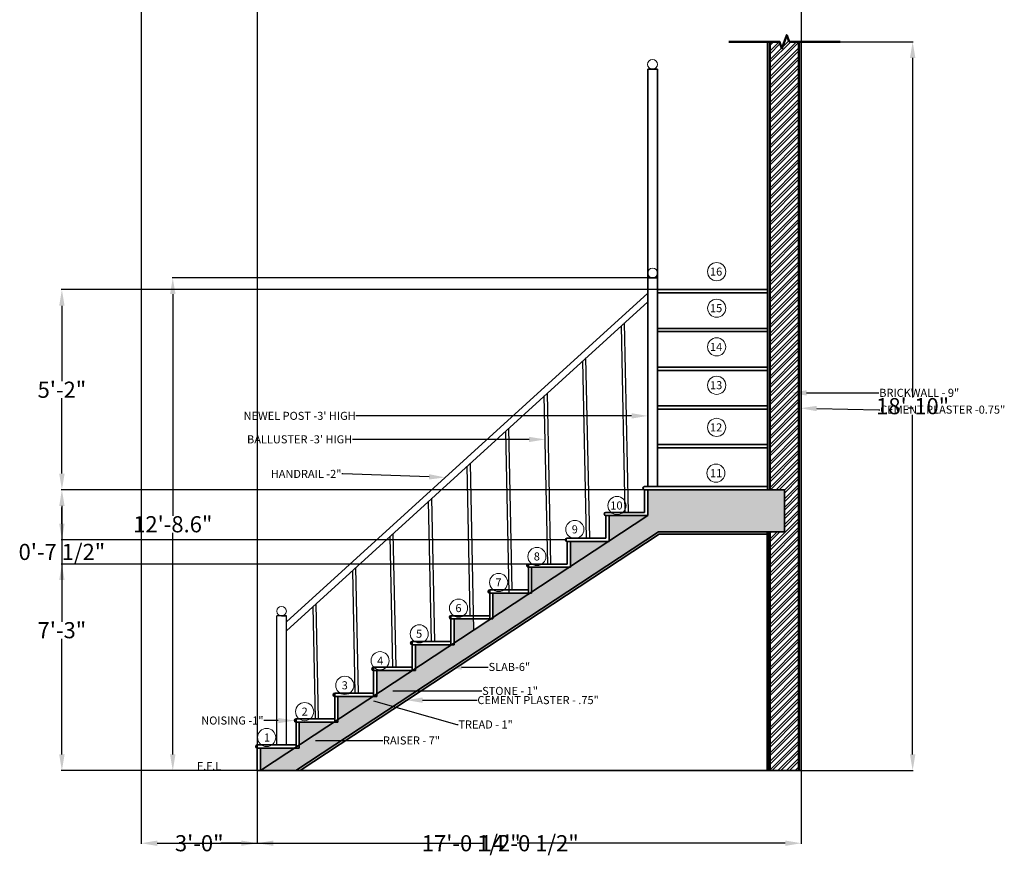
# Model space of a CAD drawing. Units: inches. Extents: x -17 to 288, y -625 to -149.
# Tile 1 of 2: x -17 to 288, y -625 to -363. Entities that reach past the tile are written whole.
import ezdxf
from ezdxf import colors
from ezdxf.entities.mleader import LeaderData, LeaderLine
from ezdxf.math import Vec2, Vec3

# ---------------------------------------------------------------- set-up
doc = ezdxf.new("R2010")
doc.units = ezdxf.units.IN
doc.header["$MEASUREMENT"] = 0
for name, color, linetype, lineweight in [('A-ANNO-DIMS', 2, 'Continuous', 18), ('A-ANNO-SYMB', 3, 'Continuous', 18), ('A-ANNO-TEXT', 7, 'Continuous', 18), ('A-FLOR-HRAL', 4, 'Continuous', 25), ('A-FLOR-PATT', 252, 'Continuous', 13), ('A-FLOR-STRS', 1, 'Continuous', 35), ('A-WALL', 7, 'Continuous', 50), ('A-WALL-PATT', 8, 'Continuous', 18)]:
    doc.layers.add(name, color=color, linetype=linetype, lineweight=lineweight)
doc.styles.get("Standard").update_dxf_attribs({"font": 'arial.ttf'})
doc.dimstyles.get("Standard").update_dxf_attribs({"dimtxt": 5, "dimasz": 5, "dimexe": 0.18, "dimexo": 0.0625, "dimgap": 0.09, "dimtad": 0, "dimtih": 1, "dimtoh": 1, "dimdec": 1, "dimzin": 0, "dimdsep": 46, "dimlunit": 3, "dimtxsty": 'Standard', "dimcen": 0, "dimadec": 0, "dimazin": 0, "dimtfac": 1, "dimtdec": 1, "dimtofl": 0, "dimtmove": 0, "dimatfit": 3, "dimfxl": 1, "dimtolj": 1, "dimtzin": 0, "dimarcsym": 1})

# ---------------------------------------------------------------- blocks, each defined once
blk = doc.blocks.new('*D4')
at = {"layer": 'A-ANNO-DIMS', "color": 0, "lineweight": -2, "transparency": 16777216}
for p, q in [((180.26, -442.5), (29.96, -442.5)), ((30.14, -447.5), (30.14, -516.18)), ((30.14, -590.14), (30.14, -521.47)), ((179.38, -595.14), (29.96, -595.14))]:
    blk.add_line(p, q, dxfattribs=at)
at = {"layer": 'A-ANNO-DIMS', "color": 0, "transparency": 16777216}
for points in [[(29.31, -447.5), (30.98, -447.5), (30.14, -442.5)], [(29.31, -590.14), (30.98, -590.14), (30.14, -595.14)]]:
    blk.add_solid(points, dxfattribs=at)
at = {"layer": 'Defpoints', "color": 0, "transparency": 16777216}
for p in [(180.32, -442.5), (30.14, -595.14), (179.44, -595.14)]:
    blk.add_point(p, dxfattribs=at)
at = {"layer": 'A-ANNO-DIMS', "color": 0, "transparency": 16777216, "insert": (30.14, -518.82), "char_height": 5, "attachment_point": 5}
blk.add_mtext('\\A1;12\'-8.6"', dxfattribs=at)
blk = doc.blocks.new('*D10')
at = {"layer": 'A-ANNO-DIMS', "color": 0, "lineweight": -2, "transparency": 16777216}
for p, q in [((20.34, -273.56), (20.34, -617.82)), ((224.91, -273.56), (224.91, -617.82)), ((25.34, -617.64), (108.36, -617.64)), ((219.91, -617.64), (136.9, -617.64))]:
    blk.add_line(p, q, dxfattribs=at)
at = {"layer": 'A-ANNO-DIMS', "color": 0, "transparency": 16777216}
for points in [[(25.34, -616.81), (25.34, -618.47), (20.34, -617.64)], [(219.91, -616.81), (219.91, -618.47), (224.91, -617.64)]]:
    blk.add_solid(points, dxfattribs=at)
at = {"layer": 'Defpoints', "color": 0, "transparency": 16777216}
for p in [(20.34, -273.5), (224.91, -273.5), (224.91, -617.64)]:
    blk.add_point(p, dxfattribs=at)
at = {"layer": 'A-ANNO-DIMS', "color": 0, "transparency": 16777216, "insert": (122.63, -617.64), "char_height": 5, "attachment_point": 5}
blk.add_mtext('\\A1;17\'-0 1/2"', dxfattribs=at)
blk = doc.blocks.new('*D12')
at = {"layer": 'A-ANNO-DIMS', "color": 0, "lineweight": -2, "transparency": 16777216}
for p, q in [((20.34, -263.06), (20.34, -617.82)), ((56.34, -263.06), (56.34, -617.82)), ((25.34, -617.64), (31.61, -617.64)), ((51.34, -617.64), (45.08, -617.64))]:
    blk.add_line(p, q, dxfattribs=at)
at = {"layer": 'A-ANNO-DIMS', "color": 0, "transparency": 16777216}
for points in [[(25.34, -616.81), (25.34, -618.47), (20.34, -617.64)], [(51.34, -616.81), (51.34, -618.47), (56.34, -617.64)]]:
    blk.add_solid(points, dxfattribs=at)
at = {"layer": 'Defpoints', "color": 0, "transparency": 16777216}
for p in [(20.34, -263), (56.34, -263), (56.34, -617.64)]:
    blk.add_point(p, dxfattribs=at)
at = {"layer": 'A-ANNO-DIMS', "color": 0, "transparency": 16777216, "insert": (38.34, -617.64), "char_height": 5, "attachment_point": 5}
blk.add_mtext('\\A1;3\'-0"', dxfattribs=at)
blk = doc.blocks.new('*D13')
at = {"layer": 'A-ANNO-DIMS', "color": 0, "lineweight": -2, "transparency": 16777216}
for p, q in [((-4.22, -518.64), (-4.22, -513.64)), ((152.28, -523.64), (-4.4, -523.64)), ((152.28, -531.14), (-4.4, -531.14)), ((-4.22, -536.14), (-4.22, -541.14))]:
    blk.add_line(p, q, dxfattribs=at)
at = {"layer": 'A-ANNO-DIMS', "color": 0, "transparency": 16777216}
for points in [[(-5.05, -518.64), (-3.38, -518.64), (-4.22, -523.64)], [(-5.05, -536.14), (-3.38, -536.14), (-4.22, -531.14)]]:
    blk.add_solid(points, dxfattribs=at)
at = {"layer": 'Defpoints', "color": 0, "transparency": 16777216}
for p in [(-4.22, -523.64), (152.34, -523.64), (152.34, -531.14)]:
    blk.add_point(p, dxfattribs=at)
at = {"layer": 'A-ANNO-DIMS', "color": 0, "transparency": 16777216, "insert": (-4.22, -527.39), "char_height": 5, "attachment_point": 5}
blk.add_mtext('\\A1;0\'-7 1/2"', dxfattribs=at)
blk = doc.blocks.new('*D14')
at = {"layer": 'A-ANNO-DIMS', "color": 0, "lineweight": -2, "transparency": 16777216}
for p, q in [((214.35, -508.14), (-4.4, -508.14)), ((-4.22, -513.14), (-4.22, -549)), ((-4.22, -590.14), (-4.22, -554.29)), ((56.28, -595.14), (-4.4, -595.14))]:
    blk.add_line(p, q, dxfattribs=at)
at = {"layer": 'A-ANNO-DIMS', "color": 0, "transparency": 16777216}
for points in [[(-5.05, -513.14), (-3.38, -513.14), (-4.22, -508.14)], [(-5.05, -590.14), (-3.38, -590.14), (-4.22, -595.14)]]:
    blk.add_solid(points, dxfattribs=at)
at = {"layer": 'Defpoints', "color": 0, "transparency": 16777216}
for p in [(-4.22, -508.14), (214.41, -508.14), (56.34, -595.14)]:
    blk.add_point(p, dxfattribs=at)
at = {"layer": 'A-ANNO-DIMS', "color": 0, "transparency": 16777216, "insert": (-4.22, -551.64), "char_height": 5, "attachment_point": 5}
blk.add_mtext('\\A1;7\'-3"', dxfattribs=at)
blk = doc.blocks.new('*D15')
at = {"layer": 'A-ANNO-DIMS', "color": 0, "lineweight": -2, "transparency": 16777216}
for p, q in [((214.35, -446.14), (-4.4, -446.14)), ((-4.22, -451.14), (-4.22, -474.5)), ((-4.22, -503.14), (-4.22, -479.78)), ((214.35, -508.14), (-4.4, -508.14))]:
    blk.add_line(p, q, dxfattribs=at)
at = {"layer": 'A-ANNO-DIMS', "color": 0, "transparency": 16777216}
for points in [[(-5.05, -451.14), (-3.38, -451.14), (-4.22, -446.14)], [(-5.05, -503.14), (-3.38, -503.14), (-4.22, -508.14)]]:
    blk.add_solid(points, dxfattribs=at)
at = {"layer": 'Defpoints', "color": 0, "transparency": 16777216}
for p in [(-4.22, -446.14), (214.41, -446.14), (214.41, -508.14)]:
    blk.add_point(p, dxfattribs=at)
at = {"layer": 'A-ANNO-DIMS', "color": 0, "transparency": 16777216, "insert": (-4.22, -477.14), "char_height": 5, "attachment_point": 5}
blk.add_mtext('\\A1;5\'-2"', dxfattribs=at)
blk = doc.blocks.new('*D16')
at = {"layer": 'A-ANNO-DIMS', "color": 0, "lineweight": -2, "transparency": 16777216}
for p, q in [((56.34, -595.2), (56.34, -617.82)), ((224.91, -595.2), (224.91, -617.82)), ((61.34, -617.64), (126.36, -617.64)), ((219.91, -617.64), (154.9, -617.64))]:
    blk.add_line(p, q, dxfattribs=at)
at = {"layer": 'A-ANNO-DIMS', "color": 0, "transparency": 16777216}
for points in [[(61.34, -616.81), (61.34, -618.47), (56.34, -617.64)], [(219.91, -616.81), (219.91, -618.47), (224.91, -617.64)]]:
    blk.add_solid(points, dxfattribs=at)
at = {"layer": 'Defpoints', "color": 0, "transparency": 16777216}
for p in [(56.34, -595.14), (224.91, -595.14), (224.91, -617.64)]:
    blk.add_point(p, dxfattribs=at)
at = {"layer": 'A-ANNO-DIMS', "color": 0, "transparency": 16777216, "insert": (140.63, -617.64), "char_height": 5, "attachment_point": 5}
blk.add_mtext('\\A1;14\'-0 1/2"', dxfattribs=at)
blk = doc.blocks.new('*D17')
at = {"layer": 'A-ANNO-DIMS', "color": 0, "lineweight": -2, "transparency": 16777216}
for p, q in [((224.98, -369.33), (259.59, -369.33)), ((259.41, -374.33), (259.41, -479.59)), ((259.41, -590.14), (259.41, -484.88)), ((224.98, -595.14), (259.59, -595.14))]:
    blk.add_line(p, q, dxfattribs=at)
at = {"layer": 'A-ANNO-DIMS', "color": 0, "transparency": 16777216}
for points in [[(258.58, -374.33), (260.25, -374.33), (259.41, -369.33)], [(258.58, -590.14), (260.25, -590.14), (259.41, -595.14)]]:
    blk.add_solid(points, dxfattribs=at)
at = {"layer": 'Defpoints', "color": 0, "transparency": 16777216}
for p in [(224.91, -369.33), (259.41, -369.33), (224.91, -595.14)]:
    blk.add_point(p, dxfattribs=at)
at = {"layer": 'A-ANNO-DIMS', "color": 0, "transparency": 16777216, "insert": (259.41, -482.23), "char_height": 5, "attachment_point": 5}
blk.add_mtext('\\A1;18\'-10"', dxfattribs=at)

msp = doc.modelspace()

# ---------------------------------------------------------------- hatches: boundary and pattern name
at = {"layer": 'A-FLOR-PATT'}
h = msp.add_hatch(dxfattribs=at)
h.set_pattern_fill('AR-CONC', color=256)
h.set_pattern_definition([(50, (-200.1796, -74.3096), (7.1726, -0.62752), [0.75, -8.25]), (355, (-200.1796, -74.3096), (-1.38751, 7.52192), [0.6, -6.6]), (100.4514, (-199.582, -74.362), (5.78509, 6.8944), [0.6374, -7.01142]), (46.1842, (-200.18, -72.31), (10.67241, -1.65519), [1.125, -12.375]), (96.6356, (-199.29, -72.448), (9.34662, 9.74119), [0.9561, -10.51714]), (351.1842, (-200.18, -72.31), (9.34662, 9.74119), [0.9, -9.9]), (21, (-199.1796, -72.8096), (5.96907, -4.02619), [0.75, -8.25]), (326, (-199.1796, -72.8096), (2.43315, 7.2515), [0.6, -6.6]), (71.4514, (-198.682, -73.145), (8.402224, 3.22531), [0.6374, -7.01142]), (37.5, (-200.1796, -74.3096), (0.121599, 3.328939), [0, -6.52, 0, -6.7, 0, -6.625]), (7.5, (-200.1796, -74.3096), (2.630695, 3.944117), [0, -3.82, 0, -6.37, 0, -2.525]), (327.5, (-202.4096, -74.3096), (5.338224, -0.225549), [0, -2.5, 0, -7.8, 0, -10.35]), (317.5, (-203.4096, -74.3096), (5.831862, 1.00105), [0, -3.25, 0, -5.18, 0, -7.35])])
h.paths.add_polyline_path([(180.64, -521.15), (219.66, -521.15), (219.66, -508.14), (188.34, -508.14), (177.34, -508.14), (177.34, -516.14), (165.34, -524.04), (165.34, -524.14), (165.19, -524.14), (153.34, -531.94), (153.34, -532.14), (153.04, -532.14), (141.34, -539.84), (141.34, -540.14), (140.89, -540.14), (129.34, -547.74), (129.34, -548.14), (128.74, -548.14), (117.34, -555.64), (117.34, -556.14), (116.58, -556.14), (105.34, -563.54), (105.34, -564.14), (104.43, -564.14), (93.34, -571.44), (93.34, -572.14), (92.28, -572.14), (81.34, -579.34), (81.34, -580.14), (80.13, -580.14), (69.34, -587.24), (69.34, -588.14), (67.98, -588.14), (57.34, -595.14), (68.26, -595.14)])
h.paths.add_polyline_path([(80.13, -580.14), (69.34, -580.14), (69.34, -587.24)], flags=17)
h.paths.add_polyline_path([(67.98, -588.14), (57.34, -588.14), (57.34, -595.14)], flags=17)
h.paths.add_polyline_path([(92.28, -572.14), (81.34, -572.14), (81.34, -579.34)], flags=17)
h.paths.add_polyline_path([(104.43, -564.14), (93.34, -564.14), (93.34, -571.44)], flags=17)
h.paths.add_polyline_path([(116.58, -556.14), (105.34, -556.14), (105.34, -563.54)], flags=17)
h.paths.add_polyline_path([(123.36, -548.14), (117.34, -548.14), (117.34, -555.64), (123.44, -551.63)], flags=17)
h.paths.add_polyline_path([(140.89, -540.14), (129.34, -540.14), (129.34, -547.74)], flags=17)
h.paths.add_polyline_path([(153.04, -532.14), (141.34, -532.14), (141.34, -539.84)], flags=17)
h.paths.add_polyline_path([(165.19, -524.14), (153.34, -524.14), (153.34, -531.94)], flags=17)
h.paths.add_polyline_path([(177.34, -516.14), (165.34, -516.14), (165.34, -524.04)], flags=17)
h.paths.add_polyline_path([(117.09, -546.71), (120.31, -546.71), (120.31, -542.88), (117.09, -542.88)], flags=25)
at = {"layer": 'A-FLOR-STRS'}
h = msp.add_hatch(dxfattribs=at)
h.set_pattern_fill('AR-CONC', color=256, scale=0.2)
h.set_pattern_definition([(50, (-200.1796, -74.3096), (1.4345204, -0.1255043), [0.15, -1.65]), (355, (-200.1796, -74.3096), (-0.2775027, 1.5043843), [0.12, -1.32]), (100.45144, (-200.06, -74.32), (1.1570177, 1.37888), [0.1274804, -1.4022842]), (46.1842, (-200.1796, -73.9096), (2.1344827, -0.3310386), [0.225, -2.475]), (96.63564, (-200.0017, -73.9372), (1.869324, 1.948237), [0.191221, -2.1034275]), (351.18416, (-200.1796, -73.9096), (1.869324, 1.948237), [0.18, -1.98]), (21, (-199.9796, -74.0096), (1.1938141, -0.8052378), [0.15, -1.65]), (326, (-199.9796, -74.0096), (0.4866307, 1.4503), [0.12, -1.32]), (71.45144, (-199.8801, -74.0767), (1.6804448, 0.6450623), [0.1274804, -1.4022842]), (37.5, (-200.1796, -74.3096), (0.0243197, 0.6657877), [0, -1.304, 0, -1.34, 0, -1.325]), (7.5, (-200.1796, -74.3096), (0.5261391, 0.7888234), [0, -0.764, 0, -1.274, 0, -0.505]), (327.5, (-200.6256, -74.3096), (1.06764487, -0.04510974), [0, -0.5, 0, -1.56, 0, -2.07]), (317.5, (-200.8256, -74.3096), (1.1663723, 0.20021), [0, -0.65, 0, -1.036, 0, -1.47])])
h.paths.add_polyline_path([(224.91, -178.83), (224.16, -178.83), (224.16, -272.75), (20.34, -272.75), (20.34, -273.5), (224.91, -273.5)])
h.paths.add_polyline_path([(224.91, -173.05), (224.91, -150.95), (224.16, -150.95), (224.16, -173.05), (224.16, -178.83), (224.91, -178.83)])
h.paths.add_polyline_path([(215.16, -173.05), (215.16, -150.95), (214.41, -150.95), (214.41, -173.05), (214.41, -263), (56.34, -263), (56.34, -263.75), (215.16, -263.75), (215.16, -263)])
h.paths.add_polyline_path([(180.87, -521.9), (214.41, -521.9), (214.41, -521.15), (180.64, -521.15), (68.34, -595.08), (68.34, -595.14), (69.62, -595.14)])
at = {"layer": 'A-WALL-PATT'}
h = msp.add_hatch(dxfattribs=at)
h.set_pattern_fill('ANSI32', color=256, scale=5)
h.set_pattern_definition([(45, (-200.1796, -74.3096), (-1.325825, 1.325825), []), (45, (-199.2957, -74.3096), (-1.325825, 1.325825), [])])
h.paths.add_polyline_path([(224.16, -369.33), (221.16, -369.33), (220.41, -367.27), (218.91, -371.39), (218.16, -369.33), (215.16, -369.33), (215.16, -508.14), (219.66, -508.14), (219.66, -521.15), (215.16, -521.15), (215.16, -595.14), (224.16, -595.14), (224.16, -508.14)])

# ---------------------------------------------------------------- linework, layer by layer
at = {"layer": 'A-ANNO-SYMB'}
for centre, radius in [((178.8, -376.34), 1.52), ((198.68, -440.56), 2.81), ((178.82, -440.98), 1.52), ((198.69, -451.89), 2.81), ((198.67, -463.86), 2.81), ((198.68, -475.76), 2.81), ((198.66, -488.81), 2.81), ((198.44, -502.99), 2.81), ((167.78, -513.02), 2.81), ((154.73, -520.42), 2.81), ((142.98, -528.81), 2.81), ((131.11, -536.85), 2.81), ((118.69, -544.8), 2.81), ((63.84, -545.74), 1.49), ((106.52, -552.78), 2.81), ((94.38, -561.1), 2.81), ((83.45, -568.72), 2.81), ((71, -576.87), 2.81), ((59.22, -584.88), 2.81)]:
    msp.add_circle(centre, radius, dxfattribs=at)
at = {"layer": 'A-FLOR-HRAL'}
for p, q in [((177.32, -441.24), (177.32, -440.72)), ((180.32, -441.24), (180.32, -440.72)), ((65.34, -549.1), (177.32, -447.19)), ((65.34, -551.8), (177.32, -449.89)), ((170.34, -515.14), (169.14, -457.34)), ((171.34, -515.12), (170.12, -456.45)), ((158.34, -523.14), (157.19, -468.21)), ((159.34, -523.12), (158.18, -467.31)), ((147.34, -531.12), (146.24, -478.18)), ((146.34, -531.14), (145.25, -479.07)), ((134.36, -540.14), (133.31, -489.94)), ((135.34, -539.14), (134.3, -489.05)), ((123.44, -551.63), (122.36, -499.91)), ((122.34, -547.14), (121.37, -500.81)), ((110.34, -555.14), (109.43, -511.67)), ((111.34, -555.12), (110.42, -510.78)), ((99.34, -563.12), (98.48, -521.65)), ((98.34, -563.14), (97.49, -522.54)), ((86.68, -571.14), (85.89, -533.1)), ((87.68, -571.14), (86.87, -532.21)), ((62.34, -545.74), (62.35, -545.74)), ((65.34, -545.74), (65.34, -545.74)), ((74.34, -579.14), (73.61, -544.27)), ((75.34, -579.12), (74.6, -543.46)), ((62.34, -551.03), (62.34, -547.23)), ((65.34, -547.23), (62.34, -547.23)), ((63.84, -547.23), (65.34, -547.23)), ((65.34, -551.14), (65.34, -547.23)), ((62.34, -587.14), (62.34, -551.03)), ((65.34, -587.14), (65.34, -551.14))]:
    msp.add_line(p, q, dxfattribs=at)
at = {"layer": 'A-FLOR-STRS'}
for p, q in [((214.41, -507.14), (214.41, -369.33)), ((224.91, -508.14), (224.91, -369.33)), ((177.3, -387.16), (177.3, -377.87)), ((180.3, -377.87), (177.3, -377.87)), ((180.3, -387.16), (180.3, -377.87)), ((177.3, -390.96), (177.3, -387.16)), ((180.3, -391.07), (180.3, -387.16)), ((177.32, -442.5), (177.32, -390.9)), ((180.3, -391.07), (180.3, -393.5)), ((180.32, -442.5), (180.32, -393.5)), ((177.32, -451.8), (177.32, -442.5)), ((180.32, -442.5), (177.32, -442.5)), ((178.82, -442.5), (180.32, -442.5)), ((180.32, -451.8), (180.32, -442.5)), ((180.32, -446.14), (214.41, -446.14)), ((180.32, -447.16), (180.34, -447.14)), ((180.34, -447.14), (214.41, -447.14)), ((177.32, -455.6), (177.32, -451.8)), ((180.32, -455.71), (180.32, -451.8)), ((177.34, -507.14), (177.34, -455.54)), ((180.32, -455.71), (180.32, -458.14)), ((180.34, -507.14), (180.34, -458.14)), ((180.34, -458.14), (214.41, -458.14)), ((180.34, -459.14), (214.41, -459.14)), ((180.34, -470.14), (214.41, -470.14)), ((180.34, -471.14), (214.41, -471.14)), ((180.34, -482.14), (214.41, -482.14)), ((180.34, -483.14), (214.41, -483.14)), ((180.34, -494.14), (214.41, -494.14)), ((180.34, -495.14), (214.41, -495.14)), ((176.34, -507.14), (214.41, -507.14)), ((176.34, -515.14), (176.34, -508.14)), ((176.34, -508.14), (188.34, -508.14)), ((177.34, -516.14), (177.34, -508.14)), ((177.34, -508.14), (177.34, -516.14)), ((188.34, -508.14), (219.66, -508.14)), ((214.41, -507.14), (214.41, -508.14)), ((219.66, -521.15), (219.66, -508.14)), ((224.91, -508.14), (224.91, -595.14)), ((164.34, -515.14), (176.34, -515.14)), ((57.34, -595.14), (177.34, -516.14)), ((164.34, -523.14), (164.34, -516.14)), ((164.34, -516.14), (177.34, -516.14)), ((165.34, -524.14), (165.34, -516.14)), ((68.26, -595.14), (180.64, -521.15)), ((180.64, -521.15), (219.66, -521.15)), ((69.62, -595.14), (180.87, -521.9)), ((152.34, -523.14), (164.34, -523.14)), ((152.34, -531.14), (152.34, -524.14)), ((152.34, -524.14), (165.34, -524.14)), ((153.34, -532.14), (153.34, -524.14)), ((180.87, -521.9), (214.41, -521.9)), ((140.34, -531.14), (140.34, -540.14)), ((140.34, -531.14), (152.34, -531.14)), ((140.34, -539.14), (140.34, -532.14)), ((140.34, -532.14), (153.34, -532.14)), ((141.34, -540.14), (141.34, -532.14)), ((128.34, -539.14), (128.34, -548.14)), ((128.34, -539.14), (140.34, -539.14)), ((128.34, -547.14), (128.34, -540.14)), ((128.34, -540.14), (141.34, -540.14)), ((129.34, -548.14), (129.34, -540.14)), ((116.34, -547.14), (116.34, -556.14)), ((116.34, -547.14), (128.34, -547.14)), ((116.34, -555.14), (116.34, -548.14)), ((116.34, -548.14), (129.34, -548.14)), ((117.34, -556.14), (117.34, -548.14)), ((104.34, -555.14), (104.34, -564.14)), ((104.34, -555.14), (116.34, -555.14)), ((104.34, -563.14), (104.34, -556.14)), ((104.34, -556.14), (117.34, -556.14)), ((105.34, -564.14), (105.34, -556.14)), ((92.34, -563.14), (92.34, -572.14)), ((92.34, -563.14), (104.34, -563.14)), ((92.34, -571.14), (92.34, -564.14)), ((92.34, -564.14), (105.34, -564.14)), ((93.34, -572.14), (93.34, -564.14)), ((80.34, -571.14), (80.34, -580.14)), ((80.34, -571.14), (92.34, -571.14)), ((80.34, -579.14), (80.34, -572.14)), ((80.34, -572.14), (93.34, -572.14)), ((81.34, -580.14), (81.34, -572.14)), ((68.34, -579.14), (68.34, -588.14)), ((68.34, -579.14), (80.34, -579.14)), ((68.34, -587.14), (68.34, -580.14)), ((68.34, -580.14), (81.34, -580.14)), ((69.34, -588.14), (69.34, -580.14)), ((56.34, -587.14), (56.34, -595.14)), ((56.34, -587.14), (68.34, -587.14)), ((56.34, -595.14), (56.34, -588.14)), ((56.34, -588.14), (69.34, -588.14)), ((57.34, -595.14), (57.34, -588.14)), ((224.91, -595.14), (56.34, -595.14)), ((68.34, -595.04), (68.34, -595.14))]:
    msp.add_line(p, q, dxfattribs=at)
for centre in [(176.34, -507.64), (164.34, -515.64), (152.34, -523.64), (140.34, -531.64), (128.34, -539.64), (116.34, -547.64), (104.34, -555.64), (92.34, -563.64), (80.34, -571.64), (68.34, -579.64), (56.34, -587.64)]:
    msp.add_arc(centre, 0.5, 90, 270, dxfattribs=at)
at = {"layer": 'A-WALL'}
for p, q in [((215.16, -508.14), (215.16, -369.33)), ((224.16, -508.14), (224.16, -369.33)), ((224.16, -508.14), (224.16, -595.14)), ((214.41, -595.14), (214.41, -521.15)), ((215.16, -595.14), (215.16, -521.15))]:
    msp.add_line(p, q, dxfattribs=at)
msp.add_lwpolyline([(202.41, -369.33), (218.16, -369.33), (218.91, -371.39), (220.41, -367.27), (221.16, -369.33), (236.91, -369.33)], dxfattribs=at)

# ---------------------------------------------------------------- texts
at = {"layer": 'A-ANNO-TEXT'}
for s, p in [('16', (196.62, -441.79)), ('15', (196.62, -453.12)), ('14', (196.62, -465.12)), ('13', (196.62, -476.99)), ('12', (196.62, -490.06)), ('11', (196.62, -504.24)), ('10', (165.73, -514.25)), ('9', (153.77, -521.65)), ('8', (142.01, -530.04)), ('7', (130.14, -538.09)), ('6', (117.73, -546.03)), ('5', (105.54, -553.99)), ('4', (93.47, -562.35)), ('3', (82.49, -569.96)), ('2', (70.07, -578.12)), ('1', (58.38, -586.14)), ('F.F.L', (37.65, -594.97))]:
    msp.add_text(s, height=2.5, dxfattribs=at).set_placement(p)

# ---------------------------------------------------------------- dimensions: what is measured, and where the dimension line sits
at = {"layer": 'A-ANNO-DIMS'}
for base, p1, p2, picture, middle in [((56.34, -617.64), (20.34, -263), (56.34, -263), '*D12', (38.34, -617.64)), ((224.91, -617.64), (20.34, -273.5), (224.91, -273.5), '*D10', (122.63, -617.64)), ((224.91, -617.64), (56.34, -595.14), (224.91, -595.14), '*D16', (140.63, -617.64))]:
    dim = msp.add_linear_dim(base=base, p1=p1, p2=p2, dimstyle='Standard', override={"dimdec": 1, "dimlfac": 1, "dimrnd": 0, "dimzin": 1, "dimdsep": 46, "dimlunit": 4, "dimfrac": 2}, dxfattribs=at)
    dim.commit()
    dim.dimension.update_dxf_attribs({"geometry": picture, "text_midpoint": middle})
for base, p1, p2, override, picture, middle in [((259.41, -369.33), (224.91, -595.14), (224.91, -369.33), {"dimdec": 1, "dimlfac": 1, "dimrnd": 0, "dimzin": 1, "dimdsep": 46, "dimlunit": 4, "dimfrac": 2}, '*D17', (259.41, -482.23)), ((30.14, -595.14), (180.32, -442.5), (179.44, -595.14), {"dimclrd": 0, "dimclre": 0, "dimclrt": 0}, '*D4', (30.14, -518.82)), ((-4.22, -446.14), (214.41, -508.14), (214.41, -446.14), {"dimdec": 1, "dimlfac": 1, "dimrnd": 0, "dimzin": 1, "dimdsep": 46, "dimlunit": 4, "dimfrac": 2}, '*D15', (-4.22, -477.14)), ((-4.22, -508.14), (56.34, -595.14), (214.41, -508.14), {"dimdec": 1, "dimlfac": 1, "dimrnd": 0, "dimzin": 1, "dimdsep": 46, "dimlunit": 4, "dimfrac": 2}, '*D14', (-4.22, -551.64)), ((-4.22, -523.64), (152.34, -531.14), (152.34, -523.64), {"dimdec": 1, "dimlfac": 1, "dimrnd": 0, "dimzin": 1, "dimdsep": 46, "dimlunit": 4, "dimfrac": 2}, '*D13', (-4.22, -527.39))]:
    dim = msp.add_linear_dim(base=base, p1=p1, p2=p2, angle=90, dimstyle='Standard', override=override, dxfattribs=at)
    dim.commit()
    dim.dimension.update_dxf_attribs({"geometry": picture, "text_midpoint": middle})

# ---------------------------------------------------------------- leaders
at = {"layer": 'A-ANNO-SYMB'}
ml = msp.add_multileader_mtext('Standard', dxfattribs=at)
ml.set_content('BRICKWALL - 9"', color=256)
ml.set_leader_properties()
ml.build(insert=Vec2(0, 0))
ml.multileader.update_dxf_attribs({"dogleg_length": 0.36, "arrow_head_size": 5})
ctx = ml.context
ctx.base_point, ctx.char_height, ctx.arrow_head_size, ctx.landing_gap_size, ctx.plane_origin = Vec3(248.97, -478.12), 2.5, 5, 0.09, Vec3(221.55, -478.12)
notes = []
notes.append((ctx, [(0, (1, 1, 0), (248.61, -478.12), (1, 0), 0.36, [(0, [(221.55, -478.12)], 0, [])])]))
ctx.mtext.insert, ctx.mtext.flow_direction = Vec3(249.06, -476.85), 5
ml = msp.add_multileader_mtext('Standard', dxfattribs=at)
ml.set_content('CEMENT PLASTER -0.75"', color=256)
ml.set_leader_properties()
ml.build(insert=Vec2(0, 0))
ml.multileader.update_dxf_attribs({"dogleg_length": 0.36, "arrow_head_size": 5})
ctx = ml.context
ctx.base_point, ctx.char_height, ctx.arrow_head_size, ctx.landing_gap_size, ctx.plane_origin = Vec3(249.27, -483.33), 2.5, 5, 0.09, Vec3(224.67, -482.87)
notes.append((ctx, [(0, (1, 1, 0), (248.91, -483.33), (1, 0), 0.36, [(0, [(224.67, -482.87)], 0, [])])]))
ctx.mtext.insert, ctx.mtext.flow_direction = Vec3(249.36, -482.06), 5
ml = msp.add_multileader_mtext('Standard', dxfattribs=at)
ml.set_content("NEWEL POST -3' HIGH", color=256)
ml.set_leader_properties()
ml.build(insert=Vec2(0, 0))
ml.multileader.update_dxf_attribs({"dogleg_length": 0.36, "arrow_head_size": 5})
ctx = ml.context
ctx.base_point, ctx.char_height, ctx.arrow_head_size, ctx.landing_gap_size, ctx.plane_origin = Vec3(49.93, -485.25), 2.5, 5, 0.09, Vec3(177.34, -485.25)
ctx.text_align_type = 2
notes.append((ctx, [(0, (1, 1, 0), (87.27, -485.25), (-1, 0), 0.36, [(0, [(177.34, -485.25)], 0, [])])]))
ctx.mtext.insert, ctx.mtext.alignment, ctx.mtext.flow_direction = Vec3(86.82, -483.98), 3, 5
ml = msp.add_multileader_mtext('Standard', dxfattribs=at)
ml.set_content("BALLUSTER -3' HIGH", color=256)
ml.set_leader_properties()
ml.build(insert=Vec2(0, 0))
ml.multileader.update_dxf_attribs({"dogleg_length": 0.36, "arrow_head_size": 5})
ctx = ml.context
ctx.base_point, ctx.char_height, ctx.arrow_head_size, ctx.landing_gap_size, ctx.plane_origin = Vec3(51.37, -492.54), 2.5, 5, 0.09, Vec3(145.54, -492.54)
ctx.text_align_type = 2
notes.append((ctx, [(0, (1, 1, 0), (86.2, -492.54), (-1, 0), 0.36, [(0, [(145.54, -492.54)], 0, [])])]))
ctx.mtext.insert, ctx.mtext.alignment, ctx.mtext.flow_direction = Vec3(85.75, -491.26), 3, 5
ml = msp.add_multileader_mtext('Standard', dxfattribs=at)
ml.set_content('HANDRAIL -2"', color=256)
ml.set_leader_properties()
ml.build(insert=Vec2(0, 0))
ml.multileader.update_dxf_attribs({"dogleg_length": 0.36, "arrow_head_size": 5})
ctx = ml.context
ctx.base_point, ctx.char_height, ctx.arrow_head_size, ctx.landing_gap_size, ctx.plane_origin = Vec3(59.79, -503.22), 2.5, 5, 0.09, Vec3(114.56, -504.31)
ctx.text_align_type = 2
notes.append((ctx, [(0, (1, 1, 0), (82.86, -503.22), (-1, 0), 0.36, [(0, [(114.56, -504.31)], 0, [])])]))
ctx.mtext.insert, ctx.mtext.alignment, ctx.mtext.flow_direction = Vec3(82.41, -501.97), 3, 5
ml = msp.add_multileader_mtext('Standard', dxfattribs=at)
ml.set_content('SLAB-6"', color=256)
ml.set_leader_properties()
ml.build(insert=Vec2(0, 0))
ml.multileader.update_dxf_attribs({"dogleg_length": 0.36, "arrow_head_size": 5})
ctx = ml.context
ctx.base_point, ctx.char_height, ctx.arrow_head_size, ctx.landing_gap_size, ctx.plane_origin = Vec3(127.91, -563.05), 2.5, 5, 0.09, Vec3(114.62, -563.05)
notes.append((ctx, [(0, (1, 1, 0), (127.55, -563.05), (1, 0), 0.36, [(0, [(114.62, -563.05)], 0, [])])]))
ctx.mtext.insert, ctx.mtext.flow_direction = Vec3(128, -561.77), 5
ml = msp.add_multileader_mtext('Standard', dxfattribs=at)
ml.set_content('STONE - 1"', color=256)
ml.set_leader_properties()
ml.build(insert=Vec2(0, 0))
ml.multileader.update_dxf_attribs({"dogleg_length": 0.36, "arrow_head_size": 5})
ctx = ml.context
ctx.base_point, ctx.char_height, ctx.arrow_head_size, ctx.landing_gap_size, ctx.plane_origin = Vec3(125.92, -570.47), 2.5, 5, 0.09, Vec3(93.34, -570.47)
notes.append((ctx, [(0, (1, 1, 0), (125.56, -570.47), (1, 0), 0.36, [(0, [(93.34, -570.47)], 0, [])])]))
ctx.mtext.insert, ctx.mtext.flow_direction = Vec3(126.01, -569.2), 5
ml = msp.add_multileader_mtext('Standard', dxfattribs=at)
ml.set_content('TREAD - 1"', color=256)
ml.set_leader_properties()
ml.build(insert=Vec2(0, 0))
ml.multileader.update_dxf_attribs({"dogleg_length": 0.36, "arrow_head_size": 5})
ctx = ml.context
ctx.base_point, ctx.char_height, ctx.arrow_head_size, ctx.landing_gap_size, ctx.plane_origin = Vec3(118.56, -580.85), 2.5, 5, 0.09, Vec3(87.55, -572.14)
notes.append((ctx, [(0, (1, 1, 0), (118.2, -580.85), (1, 0), 0.36, [(0, [(87.55, -572.14)], 0, [])])]))
ctx.mtext.insert, ctx.mtext.flow_direction = Vec3(118.65, -579.6), 5
ml = msp.add_multileader_mtext('Standard', dxfattribs=at)
ml.set_content('CEMENT PLASTER - .75"', color=256)
ml.set_leader_properties()
ml.build(insert=Vec2(0, 0))
ml.multileader.update_dxf_attribs({"dogleg_length": 0.36, "arrow_head_size": 5})
ctx = ml.context
ctx.base_point, ctx.char_height, ctx.arrow_head_size, ctx.landing_gap_size, ctx.plane_origin = Vec3(124.44, -573.31), 2.5, 5, 0.09, Vec3(102.55, -573.31)
notes.append((ctx, [(0, (1, 1, 0), (124.08, -573.31), (1, 0), 0.36, [(0, [(102.55, -573.31)], 0, [])])]))
ctx.mtext.insert, ctx.mtext.flow_direction = Vec3(124.53, -572.04), 5
ml = msp.add_multileader_mtext('Standard', dxfattribs=at)
ml.set_content('NOISING -1"', color=256)
ml.set_leader_properties()
ml.build(insert=Vec2(0, 0))
ml.multileader.update_dxf_attribs({"dogleg_length": 0.36, "arrow_head_size": 5})
ctx = ml.context
ctx.base_point, ctx.char_height, ctx.arrow_head_size, ctx.landing_gap_size, ctx.plane_origin = Vec3(38.53, -579.64), 2.5, 5, 0.09, Vec3(67.84, -579.64)
ctx.text_align_type = 2
notes.append((ctx, [(0, (1, 1, 0), (58.71, -579.64), (-1, 0), 0.36, [(0, [(67.84, -579.64)], 0, [])])]))
ctx.mtext.insert, ctx.mtext.alignment, ctx.mtext.flow_direction = Vec3(58.26, -578.37), 3, 5
ml = msp.add_multileader_mtext('Standard', dxfattribs=at)
ml.set_content('RAISER - 7"', color=256)
ml.set_leader_properties()
ml.build(insert=Vec2(0, 0))
ml.multileader.update_dxf_attribs({"dogleg_length": 0.36, "arrow_head_size": 5})
ctx = ml.context
ctx.base_point, ctx.char_height, ctx.arrow_head_size, ctx.landing_gap_size, ctx.plane_origin = Vec3(95.19, -585.82), 2.5, 5, 0.09, Vec3(69.34, -585.82)
notes.append((ctx, [(0, (1, 1, 0), (94.83, -585.82), (1, 0), 0.36, [(0, [(69.34, -585.82)], 0, [])])]))
ctx.mtext.insert, ctx.mtext.flow_direction = Vec3(95.28, -584.55), 5
for ctx, leaders in notes:
    for number, flags, end, landing, length, lines in leaders:
        leader = LeaderData()
        leader.index, (leader.has_last_leader_line, leader.has_dogleg_vector, leader.attachment_direction) = number, flags
        leader.last_leader_point, leader.dogleg_vector, leader.dogleg_length = Vec3(end), Vec3(landing), length
        for number, points, colour, breaks in lines:
            line = LeaderLine()
            line.index, line.vertices, line.color, line.breaks = number, Vec3.list(points), colors.encode_raw_color(colour), breaks
            leader.lines.append(line)
        ctx.leaders.append(leader)

doc.saveas('drawing.dxf')
